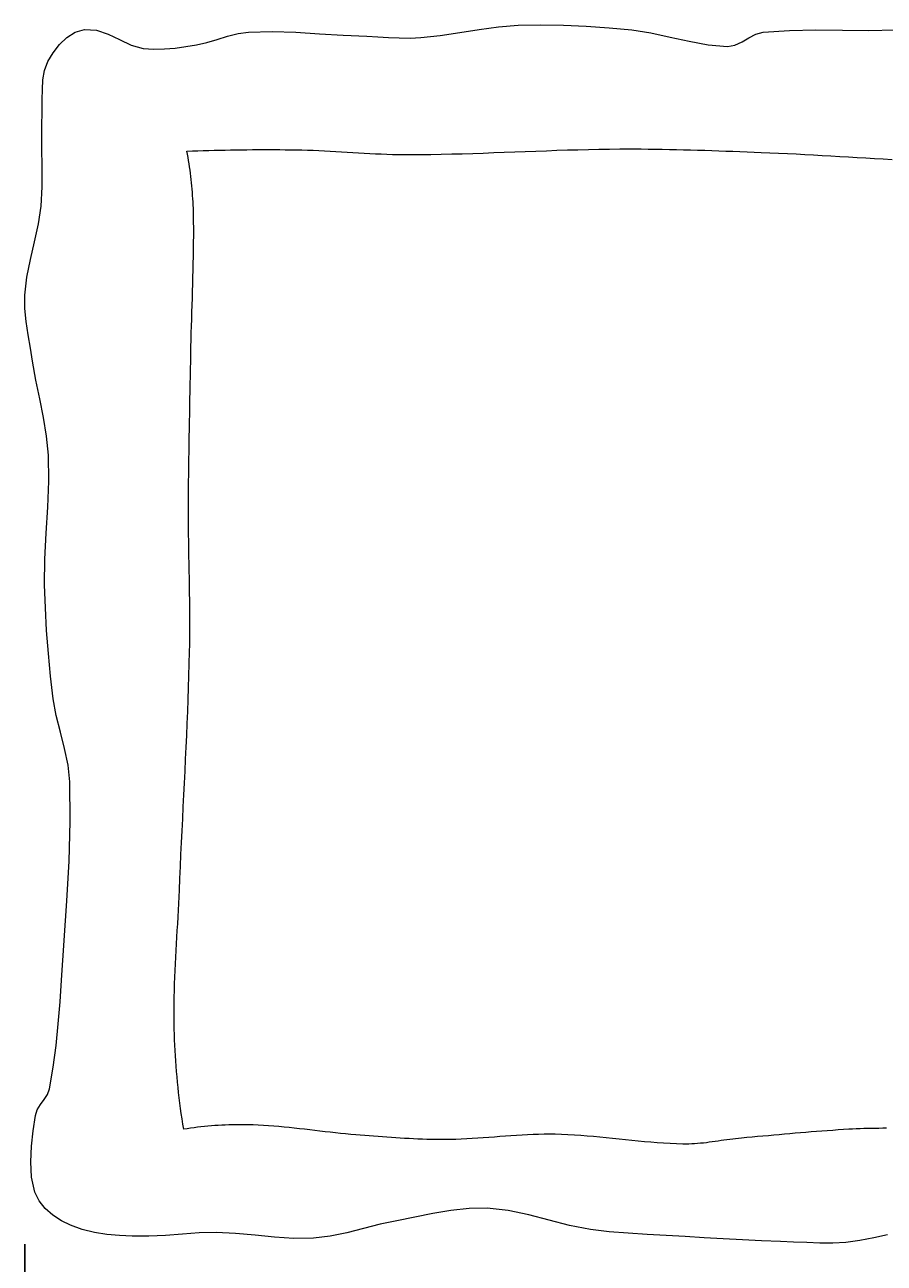
# Model space of a CAD drawing. Units: inches. Extents: x -15 to 423, y -713 to 71.
# Tile 19 of 24: x 262 to 311, y -173 to -102. Entities that reach past the tile are written whole.
import ezdxf

# ---------------------------------------------------------------- set-up
doc = ezdxf.new("R2010")
doc.units = ezdxf.units.IN
doc.header["$MEASUREMENT"] = 0
doc.layers.add('A-ANNO-DIMS', color=2, linetype='Continuous', lineweight=18)
doc.layers.add('A-FURN', color=9, linetype='Continuous', lineweight=13)
doc.styles.get("Standard").update_dxf_attribs({"font": 'arial.ttf'})
doc.dimstyles.get("Standard").update_dxf_attribs({"dimtxt": 0.18, "dimasz": 0.18, "dimexe": 0.18, "dimexo": 0.0625, "dimgap": 0.09, "dimtad": 0, "dimtih": 1, "dimtoh": 1, "dimdec": 0, "dimzin": 0, "dimdsep": 46, "dimlunit": 3, "dimtxsty": 'Standard', "dimcen": 0.09, "dimadec": 0, "dimazin": 0, "dimtfac": 1, "dimtdec": 0, "dimtofl": 0, "dimtmove": 0, "dimatfit": 3, "dimfxl": 1, "dimtolj": 1, "dimtzin": 0, "dimarcsym": 0})

# ---------------------------------------------------------------- blocks, each defined once
blk = doc.blocks.new('BED-DOUBLE')
for p, q in [((26.233, 70.103), (27.355, 70.258)), ((27.355, 70.258), (28.482, 70.345)), ((28.482, 70.345), (29.796, 70.368)), ((29.796, 70.368), (31.11, 70.346)), ((31.11, 70.346), (32.424, 70.284)), ((32.424, 70.284), (33.736, 70.19)), ((33.736, 70.19), (35.045, 70.069)), ((2.003, 69.219), (2.429, 69.63)), ((2.429, 69.63), (2.912, 69.937)), ((2.912, 69.937), (3.444, 70.1)), ((3.444, 70.1), (4.136, 70.064)), ((4.136, 70.064), (4.809, 69.832)), ((4.809, 69.832), (5.474, 69.509)), ((5.474, 69.509), (6.146, 69.198)), ((10.52, 69.337), (11.118, 69.518)), ((11.118, 69.518), (11.713, 69.708)), ((11.713, 69.708), (12.313, 69.864)), ((12.313, 69.864), (12.925, 69.947)), ((12.925, 69.947), (14.291, 69.973)), ((14.291, 69.973), (15.658, 69.932)), ((15.658, 69.932), (17.025, 69.853)), ((17.025, 69.853), (18.393, 69.767)), ((18.393, 69.767), (19.76, 69.702)), ((19.76, 69.702), (20.382, 69.674)), ((20.382, 69.674), (21.004, 69.639)), ((21.004, 69.639), (21.626, 69.611)), ((21.626, 69.611), (22.247, 69.602)), ((22.247, 69.602), (22.868, 69.627)), ((22.868, 69.627), (23.993, 69.748)), ((23.993, 69.748), (25.114, 69.92)), ((25.114, 69.92), (26.233, 70.103)), ((35.045, 70.069), (36.156, 69.9)), ((36.156, 69.9), (37.259, 69.661)), ((37.259, 69.661), (38.359, 69.412)), ((38.359, 69.412), (39.464, 69.211)), ((41.413, 69.382), (41.81, 69.617)), ((41.81, 69.617), (42.214, 69.827)), ((42.214, 69.827), (42.641, 69.942)), ((42.641, 69.942), (44.16, 70.042)), ((44.16, 70.042), (45.684, 70.067)), ((45.684, 70.067), (47.211, 70.055)), ((47.211, 70.055), (48.737, 70.043)), ((48.737, 70.043), (50.262, 70.068)), ((1.339, 68.246), (1.638, 68.744)), ((1.638, 68.744), (2.003, 69.219)), ((6.146, 69.198), (6.838, 69.007)), ((6.838, 69.007), (7.451, 68.958)), ((7.451, 68.958), (8.068, 68.97)), ((8.068, 68.97), (8.686, 69.026)), ((8.686, 69.026), (9.302, 69.109)), ((9.302, 69.109), (9.914, 69.204)), ((9.914, 69.204), (10.52, 69.337)), ((39.464, 69.211), (40.58, 69.118)), ((40.58, 69.118), (41.008, 69.192)), ((41.008, 69.192), (41.413, 69.382)), ((1.142, 67.735), (1.339, 68.246)), ((1.045, 67.191), (1.142, 67.735)), ((1.011, 66.057), (1.014, 66.627)), ((1.014, 66.627), (1.045, 67.191)), ((1, 65.495), (1.011, 66.057)), ((0.976, 64.376), (1, 65.495)), ((0.991, 63.255), (0.976, 64.376)), ((1.011, 62.135), (0.991, 63.255)), ((9.366, 63.066), (9.681, 63.078)), ((9.399, 62.885), (9.366, 63.066)), ((9.681, 63.078), (9.995, 63.09)), ((9.995, 63.09), (10.31, 63.1)), ((10.31, 63.1), (10.625, 63.11)), ((10.625, 63.11), (10.94, 63.119)), ((10.94, 63.119), (11.255, 63.127)), ((11.255, 63.127), (11.57, 63.134)), ((11.57, 63.134), (11.885, 63.14)), ((11.885, 63.14), (12.2, 63.145)), ((12.2, 63.145), (12.515, 63.15)), ((12.515, 63.15), (12.83, 63.153)), ((12.83, 63.153), (13.145, 63.156)), ((13.145, 63.156), (13.46, 63.158)), ((13.46, 63.158), (13.775, 63.159)), ((13.775, 63.159), (14.09, 63.159)), ((14.09, 63.159), (14.405, 63.158)), ((14.405, 63.158), (14.72, 63.156)), ((14.72, 63.156), (15.035, 63.154)), ((15.035, 63.154), (15.35, 63.15)), ((15.35, 63.15), (15.665, 63.146)), ((15.665, 63.146), (15.993, 63.139)), ((15.993, 63.139), (16.321, 63.13)), ((16.321, 63.13), (16.649, 63.118)), ((16.649, 63.118), (16.978, 63.104)), ((16.978, 63.104), (17.306, 63.088)), ((17.306, 63.088), (17.634, 63.07)), ((17.634, 63.07), (17.962, 63.052)), ((17.962, 63.052), (18.29, 63.032)), ((18.29, 63.032), (18.618, 63.013)), ((18.618, 63.013), (18.946, 62.993)), ((18.946, 62.993), (19.274, 62.973)), ((19.274, 62.973), (19.602, 62.954)), ((19.602, 62.954), (19.93, 62.937)), ((25.868, 62.94), (26.475, 62.96)), ((26.475, 62.96), (27.081, 62.982)), ((27.081, 62.982), (27.688, 63.004)), ((27.688, 63.004), (28.295, 63.027)), ((28.295, 63.027), (28.901, 63.05)), ((28.901, 63.05), (29.508, 63.073)), ((29.508, 63.073), (30.115, 63.095)), ((30.115, 63.095), (30.721, 63.116)), ((30.721, 63.116), (31.328, 63.135)), ((31.328, 63.135), (31.935, 63.153)), ((31.935, 63.153), (32.542, 63.168)), ((32.542, 63.168), (33.148, 63.181)), ((33.148, 63.181), (33.755, 63.19)), ((33.755, 63.19), (34.362, 63.196)), ((34.362, 63.196), (34.77, 63.197)), ((34.77, 63.197), (35.178, 63.197)), ((35.178, 63.197), (35.586, 63.195)), ((35.586, 63.195), (35.994, 63.192)), ((35.994, 63.192), (36.402, 63.187)), ((36.402, 63.187), (36.81, 63.18)), ((36.81, 63.18), (37.218, 63.172)), ((37.218, 63.172), (37.626, 63.163)), ((37.626, 63.163), (38.034, 63.153)), ((38.034, 63.153), (38.442, 63.142)), ((38.442, 63.142), (38.85, 63.13)), ((38.85, 63.13), (39.258, 63.117)), ((39.258, 63.117), (39.666, 63.103)), ((39.666, 63.103), (40.073, 63.089)), ((40.073, 63.089), (40.481, 63.074)), ((40.481, 63.074), (40.889, 63.059)), ((40.889, 63.059), (41.297, 63.044)), ((41.297, 63.044), (41.705, 63.028)), ((41.705, 63.028), (42.112, 63.013)), ((42.112, 63.013), (42.52, 62.997)), ((42.52, 62.997), (43.024, 62.977)), ((43.024, 62.977), (43.528, 62.954)), ((43.528, 62.954), (44.032, 62.93)), ((9.431, 62.703), (9.399, 62.885)), ((9.461, 62.522), (9.431, 62.703)), ((9.49, 62.34), (9.461, 62.522)), ((9.518, 62.157), (9.49, 62.34)), ((19.93, 62.937), (20.258, 62.92)), ((20.258, 62.92), (20.586, 62.905)), ((20.586, 62.905), (20.914, 62.893)), ((20.914, 62.893), (21.242, 62.882)), ((21.242, 62.882), (21.57, 62.875)), ((21.57, 62.875), (21.899, 62.87)), ((21.899, 62.87), (22.227, 62.869)), ((22.227, 62.869), (22.834, 62.873)), ((22.834, 62.873), (23.441, 62.88)), ((23.441, 62.88), (24.048, 62.891)), ((24.048, 62.891), (24.654, 62.905)), ((24.654, 62.905), (25.261, 62.921)), ((25.261, 62.921), (25.868, 62.94)), ((44.032, 62.93), (44.535, 62.904)), ((44.535, 62.904), (45.039, 62.877)), ((45.039, 62.877), (45.543, 62.849)), ((45.543, 62.849), (46.046, 62.82)), ((46.046, 62.82), (46.55, 62.791)), ((46.55, 62.791), (47.053, 62.762)), ((47.053, 62.762), (47.557, 62.732)), ((47.557, 62.732), (48.06, 62.703)), ((48.06, 62.703), (48.564, 62.675)), ((48.564, 62.675), (49.068, 62.647)), ((49.068, 62.647), (49.571, 62.62)), ((49.571, 62.62), (50.075, 62.595)), ((1.006, 61.015), (1.011, 62.135)), ((9.543, 61.975), (9.518, 62.157)), ((9.568, 61.792), (9.543, 61.975)), ((9.59, 61.609), (9.568, 61.792)), ((9.612, 61.426), (9.59, 61.609)), ((0.942, 59.899), (1.006, 61.015)), ((9.631, 61.242), (9.612, 61.426)), ((9.649, 61.059), (9.631, 61.242)), ((9.666, 60.875), (9.649, 61.059)), ((9.681, 60.691), (9.666, 60.875)), ((9.694, 60.507), (9.681, 60.691)), ((9.706, 60.323), (9.694, 60.507)), ((9.717, 60.139), (9.706, 60.323)), ((9.726, 59.955), (9.717, 60.139)), ((0.791, 58.864), (0.942, 59.899)), ((9.733, 59.771), (9.726, 59.955)), ((9.739, 59.587), (9.733, 59.771)), ((9.743, 59.403), (9.739, 59.587)), ((9.749, 59.001), (9.743, 59.403)), ((0.568, 57.839), (0.791, 58.864)), ((9.752, 58.599), (9.749, 59.001)), ((9.751, 57.794), (9.753, 58.197)), ((9.753, 58.197), (9.752, 58.599)), ((0.326, 56.816), (0.568, 57.839)), ((9.74, 56.99), (9.746, 57.392)), ((9.746, 57.392), (9.751, 57.794)), ((0.119, 55.79), (0.326, 56.816)), ((9.723, 56.186), (9.732, 56.588)), ((9.732, 56.588), (9.74, 56.99)), ((9.713, 55.784), (9.723, 56.186)), ((0, 54.752), (0.119, 55.79)), ((9.689, 54.98), (9.701, 55.382)), ((9.701, 55.382), (9.713, 55.784)), ((0.002, 53.985), (0, 54.752)), ((9.663, 54.176), (9.676, 54.578)), ((9.676, 54.578), (9.689, 54.98)), ((0.074, 53.22), (0.002, 53.985)), ((9.637, 53.371), (9.65, 53.773)), ((9.65, 53.773), (9.663, 54.176)), ((0.191, 52.456), (0.074, 53.22)), ((9.614, 52.567), (9.625, 52.969)), ((9.625, 52.969), (9.637, 53.371)), ((0.325, 51.694), (0.191, 52.456)), ((9.603, 52.165), (9.614, 52.567)), ((0.451, 50.932), (0.325, 51.694)), ((9.586, 51.361), (9.594, 51.763)), ((9.594, 51.763), (9.603, 52.165)), ((0.64, 49.847), (0.451, 50.932)), ((9.571, 50.49), (9.579, 50.926)), ((9.579, 50.926), (9.586, 51.361)), ((9.562, 50.055), (9.571, 50.49)), ((0.862, 48.766), (0.64, 49.847)), ((9.546, 49.185), (9.554, 49.62)), ((9.554, 49.62), (9.562, 50.055)), ((1.08, 47.685), (0.862, 48.766)), ((9.529, 48.315), (9.537, 48.75)), ((9.537, 48.75), (9.546, 49.185)), ((9.521, 47.879), (9.529, 48.315)), ((1.261, 46.6), (1.08, 47.685)), ((9.505, 47.009), (9.512, 47.444)), ((9.512, 47.444), (9.521, 47.879)), ((1.369, 45.507), (1.261, 46.6)), ((9.49, 46.139), (9.497, 46.574)), ((9.497, 46.574), (9.505, 47.009)), ((9.483, 45.704), (9.49, 46.139)), ((1.392, 44.009), (1.369, 45.507)), ((9.471, 44.833), (9.477, 45.268)), ((9.477, 45.268), (9.483, 45.704)), ((9.461, 43.963), (9.466, 44.398)), ((9.466, 44.398), (9.471, 44.833)), ((1.334, 42.51), (1.392, 44.009)), ((9.457, 43.528), (9.461, 43.963)), ((9.452, 42.657), (9.454, 43.092)), ((9.454, 43.092), (9.457, 43.528)), ((1.242, 41.01), (1.334, 42.51)), ((9.451, 42.232), (9.452, 42.657)), ((9.453, 41.806), (9.451, 42.232)), ((9.456, 41.38), (9.453, 41.806)), ((1.164, 39.51), (1.242, 41.01)), ((9.461, 40.954), (9.456, 41.38)), ((9.467, 40.529), (9.461, 40.954)), ((9.474, 40.103), (9.467, 40.529)), ((9.481, 39.677), (9.474, 40.103)), ((1.147, 38.01), (1.164, 39.51)), ((9.489, 39.251), (9.481, 39.677)), ((9.497, 38.826), (9.489, 39.251)), ((9.505, 38.4), (9.497, 38.826)), ((1.189, 36.691), (1.147, 38.01)), ((9.513, 37.974), (9.505, 38.4)), ((9.519, 37.548), (9.513, 37.974)), ((9.525, 37.123), (9.519, 37.548)), ((1.262, 35.372), (1.189, 36.691)), ((9.53, 36.697), (9.525, 37.123)), ((9.533, 36.271), (9.53, 36.697)), ((9.535, 35.846), (9.533, 36.271)), ((9.534, 35.42), (9.535, 35.846)), ((1.364, 34.055), (1.262, 35.372)), ((9.531, 34.994), (9.534, 35.42)), ((9.517, 34.143), (9.525, 34.569)), ((9.525, 34.569), (9.531, 34.994)), ((1.493, 32.741), (1.364, 34.055)), ((9.499, 33.455), (9.517, 34.143)), ((9.479, 32.766), (9.499, 33.455)), ((1.648, 31.429), (1.493, 32.741)), ((9.457, 32.078), (9.479, 32.766)), ((9.433, 31.389), (9.457, 32.078)), ((1.821, 30.468), (1.648, 31.429)), ((9.406, 30.701), (9.433, 31.389)), ((2.058, 29.516), (1.821, 30.468)), ((9.378, 30.012), (9.406, 30.701)), ((2.303, 28.566), (2.058, 29.516)), ((9.349, 29.324), (9.378, 30.012)), ((9.286, 27.948), (9.318, 28.636)), ((9.318, 28.636), (9.349, 29.324)), ((2.502, 27.612), (2.303, 28.566)), ((9.254, 27.26), (9.286, 27.948)), ((2.6, 26.645), (2.502, 27.612)), ((9.221, 26.572), (9.254, 27.26)), ((2.618, 24.352), (2.6, 26.645)), ((9.187, 25.883), (9.221, 26.572)), ((9.153, 25.195), (9.187, 25.883)), ((9.12, 24.507), (9.153, 25.195)), ((2.555, 22.06), (2.618, 24.352)), ((9.086, 23.819), (9.12, 24.507)), ((9.053, 23.131), (9.086, 23.819)), ((9.02, 22.443), (9.053, 23.131)), ((8.989, 21.755), (9.02, 22.443)), ((2.435, 19.769), (2.555, 22.06)), ((8.958, 21.066), (8.989, 21.755)), ((8.929, 20.378), (8.958, 21.066)), ((8.912, 19.992), (8.929, 20.378)), ((2.283, 17.478), (2.435, 19.769)), ((8.873, 19.219), (8.893, 19.606)), ((8.893, 19.606), (8.912, 19.992)), ((8.83, 18.447), (8.852, 18.833)), ((8.852, 18.833), (8.873, 19.219)), ((8.785, 17.674), (8.807, 18.06)), ((8.807, 18.06), (8.83, 18.447)), ((2.127, 15.19), (2.283, 17.478)), ((8.74, 16.901), (8.762, 17.288)), ((8.762, 17.288), (8.785, 17.674)), ((8.699, 16.129), (8.719, 16.515)), ((8.719, 16.515), (8.74, 16.901)), ((8.664, 15.356), (8.681, 15.742)), ((8.681, 15.742), (8.699, 16.129)), ((2.039, 13.928), (2.127, 15.19)), ((8.649, 14.97), (8.664, 15.356)), ((8.628, 14.197), (8.637, 14.583)), ((8.637, 14.583), (8.649, 14.97)), ((1.937, 12.667), (2.039, 13.928)), ((8.619, 13.424), (8.622, 13.81)), ((8.622, 13.81), (8.628, 14.197)), ((8.619, 13.037), (8.619, 13.424)), ((8.624, 12.651), (8.619, 13.037)), ((1.808, 11.408), (1.937, 12.667)), ((8.631, 12.346), (8.624, 12.651)), ((8.64, 12.04), (8.631, 12.346)), ((8.651, 11.735), (8.64, 12.04)), ((8.664, 11.43), (8.651, 11.735)), ((1.642, 10.155), (1.808, 11.408)), ((8.679, 11.125), (8.664, 11.43)), ((8.697, 10.82), (8.679, 11.125)), ((8.717, 10.516), (8.697, 10.82)), ((1.43, 8.91), (1.642, 10.155)), ((8.739, 10.211), (8.717, 10.516)), ((8.763, 9.906), (8.739, 10.211)), ((8.79, 9.602), (8.763, 9.906)), ((8.818, 9.298), (8.79, 9.602)), ((1.119, 8.289), (1.31, 8.587)), ((1.31, 8.587), (1.43, 8.91)), ((8.849, 8.994), (8.818, 9.298)), ((8.883, 8.69), (8.849, 8.994)), ((8.918, 8.387), (8.883, 8.69)), ((0.72, 7.7), (0.905, 7.999)), ((0.905, 7.999), (1.119, 8.289)), ((8.955, 8.084), (8.918, 8.387)), ((8.995, 7.781), (8.955, 8.084)), ((0.489, 6.488), (0.615, 7.375)), ((0.615, 7.375), (0.72, 7.7)), ((9.037, 7.479), (8.995, 7.781)), ((9.081, 7.176), (9.037, 7.479)), ((9.127, 6.875), (9.081, 7.176)), ((0.386, 5.589), (0.489, 6.488)), ((9.176, 6.573), (9.127, 6.875)), ((9.374, 6.604), (9.176, 6.573)), ((9.573, 6.633), (9.374, 6.604)), ((9.773, 6.66), (9.573, 6.633)), ((9.972, 6.685), (9.773, 6.66)), ((10.172, 6.708), (9.972, 6.685)), ((10.372, 6.729), (10.172, 6.708)), ((10.573, 6.748), (10.372, 6.729)), ((10.773, 6.766), (10.573, 6.748)), ((10.974, 6.781), (10.773, 6.766)), ((11.175, 6.795), (10.974, 6.781)), ((11.376, 6.806), (11.175, 6.795)), ((11.577, 6.816), (11.376, 6.806)), ((11.778, 6.824), (11.577, 6.816)), ((11.979, 6.83), (11.778, 6.824)), ((12.18, 6.834), (11.979, 6.83)), ((12.382, 6.836), (12.18, 6.834)), ((12.583, 6.836), (12.382, 6.836)), ((12.784, 6.835), (12.583, 6.836)), ((12.985, 6.831), (12.784, 6.835)), ((13.186, 6.826), (12.985, 6.831)), ((13.483, 6.814), (13.186, 6.826)), ((13.781, 6.798), (13.483, 6.814)), ((14.078, 6.779), (13.781, 6.798)), ((14.375, 6.756), (14.078, 6.779)), ((14.672, 6.731), (14.375, 6.756)), ((14.969, 6.703), (14.672, 6.731)), ((15.265, 6.673), (14.969, 6.703)), ((15.561, 6.641), (15.265, 6.673)), ((15.858, 6.607), (15.561, 6.641)), ((16.154, 6.573), (15.858, 6.607)), ((16.45, 6.538), (16.154, 6.573)), ((16.746, 6.503), (16.45, 6.538)), ((17.043, 6.467), (16.746, 6.503)), ((17.339, 6.432), (17.043, 6.467)), ((45.72, 6.441), (45.41, 6.416)), ((46.029, 6.465), (45.72, 6.441)), ((46.339, 6.488), (46.029, 6.465)), ((46.649, 6.51), (46.339, 6.488)), ((46.959, 6.532), (46.649, 6.51)), ((47.269, 6.552), (46.959, 6.532)), ((47.579, 6.571), (47.269, 6.552)), ((47.797, 6.583), (47.579, 6.571)), ((48.014, 6.593), (47.797, 6.583)), ((48.232, 6.602), (48.014, 6.593)), ((48.45, 6.608), (48.232, 6.602)), ((48.668, 6.614), (48.45, 6.608)), ((48.886, 6.618), (48.668, 6.614)), ((49.104, 6.622), (48.886, 6.618)), ((49.322, 6.624), (49.104, 6.622)), ((49.54, 6.627), (49.322, 6.624)), ((49.758, 6.629), (49.54, 6.627)), ((17.635, 6.398), (17.339, 6.432)), ((17.932, 6.366), (17.635, 6.398)), ((18.228, 6.334), (17.932, 6.366)), ((18.525, 6.305), (18.228, 6.334)), ((18.822, 6.278), (18.525, 6.305)), ((19.119, 6.254), (18.822, 6.278)), ((19.375, 6.234), (19.119, 6.254)), ((19.63, 6.214), (19.375, 6.234)), ((19.886, 6.194), (19.63, 6.214)), ((20.142, 6.174), (19.886, 6.194)), ((20.398, 6.154), (20.142, 6.174)), ((20.654, 6.134), (20.398, 6.154)), ((20.91, 6.115), (20.654, 6.134)), ((21.166, 6.097), (20.91, 6.115)), ((21.423, 6.079), (21.166, 6.097)), ((21.679, 6.062), (21.423, 6.079)), ((21.935, 6.047), (21.679, 6.062)), ((22.191, 6.032), (21.935, 6.047)), ((22.448, 6.019), (22.191, 6.032)), ((22.704, 6.007), (22.448, 6.019)), ((22.96, 5.997), (22.704, 6.007)), ((23.217, 5.988), (22.96, 5.997)), ((23.473, 5.981), (23.217, 5.988)), ((23.73, 5.977), (23.473, 5.981)), ((23.986, 5.974), (23.73, 5.977)), ((24.243, 5.973), (23.986, 5.974)), ((24.562, 5.977), (24.243, 5.973)), ((24.881, 5.985), (24.562, 5.977)), ((25.201, 5.996), (24.881, 5.985)), ((25.52, 6.012), (25.201, 5.996)), ((25.839, 6.03), (25.52, 6.012)), ((26.158, 6.051), (25.839, 6.03)), ((26.477, 6.073), (26.158, 6.051)), ((26.796, 6.097), (26.477, 6.073)), ((27.115, 6.121), (26.796, 6.097)), ((27.434, 6.146), (27.115, 6.121)), ((27.753, 6.17), (27.434, 6.146)), ((28.072, 6.194), (27.753, 6.17)), ((28.391, 6.216), (28.072, 6.194)), ((28.71, 6.236), (28.391, 6.216)), ((29.029, 6.253), (28.71, 6.236)), ((29.348, 6.268), (29.029, 6.253)), ((29.667, 6.279), (29.348, 6.268)), ((29.986, 6.286), (29.667, 6.279)), ((30.305, 6.288), (29.986, 6.286)), ((30.625, 6.284), (30.305, 6.288)), ((30.994, 6.274), (30.625, 6.284)), ((31.364, 6.259), (30.994, 6.274)), ((31.732, 6.238), (31.364, 6.259)), ((32.101, 6.213), (31.732, 6.238)), ((32.47, 6.183), (32.101, 6.213)), ((32.838, 6.151), (32.47, 6.183)), ((33.206, 6.116), (32.838, 6.151)), ((33.574, 6.079), (33.206, 6.116)), ((33.943, 6.041), (33.574, 6.079)), ((34.311, 6.002), (33.943, 6.041)), ((34.679, 5.963), (34.311, 6.002)), ((35.047, 5.925), (34.679, 5.963)), ((35.415, 5.888), (35.047, 5.925)), ((35.783, 5.853), (35.415, 5.888)), ((36.152, 5.82), (35.783, 5.853)), ((36.52, 5.791), (36.152, 5.82)), ((36.889, 5.765), (36.52, 5.791)), ((37.258, 5.743), (36.889, 5.765)), ((37.627, 5.727), (37.258, 5.743)), ((37.996, 5.716), (37.627, 5.727)), ((38.507, 5.724), (38.337, 5.717)), ((38.676, 5.733), (38.507, 5.724)), ((38.846, 5.746), (38.676, 5.733)), ((39.016, 5.761), (38.846, 5.746)), ((39.185, 5.779), (39.016, 5.761)), ((39.354, 5.798), (39.185, 5.779)), ((39.524, 5.82), (39.354, 5.798)), ((39.693, 5.842), (39.524, 5.82)), ((39.862, 5.865), (39.693, 5.842)), ((40.031, 5.889), (39.862, 5.865)), ((40.201, 5.914), (40.031, 5.889)), ((40.37, 5.938), (40.201, 5.914)), ((40.539, 5.961), (40.37, 5.938)), ((40.708, 5.984), (40.539, 5.961)), ((40.878, 6.006), (40.708, 5.984)), ((41.047, 6.026), (40.878, 6.006)), ((41.217, 6.045), (41.047, 6.026)), ((41.386, 6.061), (41.217, 6.045)), ((41.696, 6.089), (41.386, 6.061)), ((42.005, 6.117), (41.696, 6.089)), ((42.315, 6.145), (42.005, 6.117)), ((42.624, 6.173), (42.315, 6.145)), ((42.934, 6.201), (42.624, 6.173)), ((43.243, 6.229), (42.934, 6.201)), ((43.552, 6.257), (43.243, 6.229)), ((43.862, 6.284), (43.552, 6.257)), ((44.171, 6.312), (43.862, 6.284)), ((44.481, 6.338), (44.171, 6.312)), ((44.791, 6.365), (44.481, 6.338)), ((45.1, 6.391), (44.791, 6.365)), ((45.41, 6.416), (45.1, 6.391)), ((0.342, 4.691), (0.386, 5.589)), ((38.167, 5.715), (37.996, 5.716)), ((38.337, 5.717), (38.167, 5.715)), ((0.396, 3.805), (0.342, 4.691)), ((0.585, 2.944), (0.396, 3.805)), ((0.826, 2.44), (0.585, 2.944)), ((1.185, 1.996), (0.826, 2.44)), ((1.628, 1.613), (1.185, 1.996)), ((2.124, 1.291), (1.628, 1.613)), ((22.516, 1.488), (21.476, 1.289)), ((23.558, 1.698), (22.516, 1.488)), ((24.602, 1.881), (23.558, 1.698)), ((25.65, 2), (24.602, 1.881)), ((26.702, 2.017), (25.65, 2)), ((27.907, 1.881), (26.702, 2.017)), ((29.096, 1.626), (27.907, 1.881)), ((30.278, 1.316), (29.096, 1.626)), ((2.637, 1.029), (2.124, 1.291)), ((3.313, 0.777), (2.637, 1.029)), ((4.018, 0.609), (3.313, 0.777)), ((19.558, 0.843), (18.603, 0.6)), ((20.513, 1.087), (19.558, 0.843)), ((21.476, 1.289), (20.513, 1.087)), ((31.462, 1.013), (30.278, 1.316)), ((32.658, 0.783), (31.462, 1.013)), ((33.747, 0.653), (32.658, 0.783)), ((4.74, 0.502), (4.018, 0.609)), ((5.471, 0.439), (4.74, 0.502)), ((6.198, 0.398), (5.471, 0.439)), ((7.166, 0.391), (6.198, 0.398)), ((8.135, 0.443), (7.166, 0.391)), ((9.104, 0.52), (8.135, 0.443)), ((10.073, 0.587), (9.104, 0.52)), ((11.042, 0.61), (10.073, 0.587)), ((12.169, 0.556), (11.042, 0.61)), ((13.295, 0.449), (12.169, 0.556)), ((14.42, 0.337), (13.295, 0.449)), ((15.545, 0.264), (14.42, 0.337)), ((16.67, 0.279), (15.545, 0.264)), ((17.642, 0.398), (16.67, 0.279)), ((18.603, 0.6), (17.642, 0.398)), ((34.84, 0.562), (33.747, 0.653)), ((35.936, 0.496), (34.84, 0.562)), ((37.033, 0.44), (35.936, 0.496)), ((38.129, 0.378), (37.033, 0.44)), ((39.231, 0.31), (38.129, 0.378)), ((40.333, 0.246), (39.231, 0.31)), ((41.435, 0.186), (40.333, 0.246)), ((42.538, 0.134), (41.435, 0.186)), ((43.641, 0.088), (42.538, 0.134)), ((44.395, 0.056), (43.641, 0.088)), ((45.149, 0.023), (44.395, 0.056)), ((45.904, 0), (45.149, 0.023)), ((46.658, 0), (45.904, 0)), ((47.41, 0.036), (46.658, 0)), ((48.217, 0.14), (47.41, 0.036)), ((49.019, 0.3), (48.217, 0.14)), ((49.818, 0.473), (49.019, 0.3))]:
    blk.add_line(p, q)
blk = doc.blocks.new('*D31')
at = {"layer": 'A-ANNO-DIMS', "color": 0, "lineweight": -2, "transparency": 16777216}
for p, q in [((261.638, -171.991), (261.638, -187.148)), ((361.906, -171.991), (361.906, -187.148)), ((261.818, -186.968), (310.634, -186.968)), ((361.726, -186.968), (312.91, -186.968))]:
    blk.add_line(p, q, dxfattribs=at)
at = {"layer": 'A-ANNO-DIMS', "color": 0, "transparency": 16777216}
for points in [[(261.818, -186.938), (261.818, -186.998), (261.638, -186.968)], [(361.726, -186.938), (361.726, -186.998), (361.906, -186.968)]]:
    blk.add_solid(points, dxfattribs=at)
at = {"layer": 'Defpoints', "color": 0, "transparency": 16777216}
for p in [(261.638, -171.928), (361.906, -171.928), (361.906, -186.968)]:
    blk.add_point(p, dxfattribs=at)
at = {"layer": 'A-ANNO-DIMS', "color": 0, "transparency": 16777216, "insert": (311.772, -186.968), "char_height": 0.18, "attachment_point": 5}
blk.add_mtext('\\A1;BED 8\'-4 1/2" TYP.', dxfattribs=at)

msp = doc.modelspace()

# ---------------------------------------------------------------- block references
at = {"layer": 'A-FURN'}
msp.add_blockref('BED-DOUBLE', (261.638, -171.928), dxfattribs=at)

# ---------------------------------------------------------------- dimensions: what is measured, and where the dimension line sits
at = {"layer": 'A-ANNO-DIMS'}
dim = msp.add_linear_dim(base=(361.906, -186.968), p1=(261.638, -171.928), p2=(361.906, -171.928), text='BED <> TYP.', dimstyle='Standard', override={"dimdec": 1, "dimlfac": 1, "dimrnd": 0, "dimzin": 1, "dimdsep": 46, "dimlunit": 4, "dimfrac": 2}, dxfattribs=at)
dim.commit()
dim.dimension.update_dxf_attribs({"geometry": '*D31', "text_midpoint": (311.772, -186.968)})

doc.saveas('drawing.dxf')
